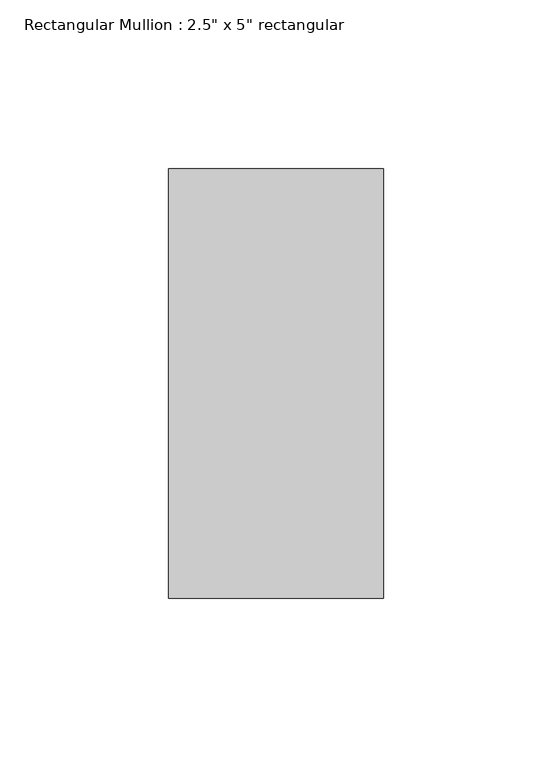
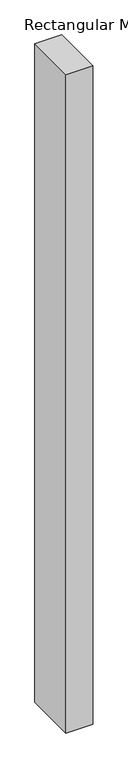
"""IFC4 building model written with IfcOpenShell, lengths in millimetres: member geometry."""

from ifc_helpers import new_model, si_unit, frame, origin, place, context, project, spatial, polyline, outline, extrude, source, transform, mapped, element, save


def member_61c652d3(model_context):
    return source(origin(), model_context, "Body", "SweptSolid", [
        extrude(outline(polyline([(0.0, 63.5), (0.0, -63.5), (-63.5, -63.5), (-63.5, 63.5), (0.0, 63.5)])), frame((0.0, 0.0, -1645.1858302), z_axis=(0.0, 0.0, 1.0), x_axis=(1.0, 0.0, 0.0)), (0.0, 0.0, 1.0), 1645.1858302),
    ])


if __name__ == "__main__":
    model = new_model("IFC4")
    model_context = context("Model", 3, world=origin())
    ifc_project = project(units=[si_unit("LENGTHUNIT", "METRE", prefix="MILLI")], contexts=[model_context])
    site = spatial("IfcSite", under=ifc_project)
    building = spatial("IfcBuilding", under=site)
    placement = place(None, origin())
    member_shape = member_61c652d3(model_context)
    element("IfcMember", 1, ObjectType="Rectangular Mullion : 2.5\" x 5\" rectangular", at=placement, inside=building, context=model_context, shape_type="MappedRepresentation", body=[
        mapped(member_shape, transform((0.0, 0.0, 0.0), x_axis=(1.0, 0.0, 0.0), y_axis=(0.0, 1.0, 0.0), z_axis=(0.0, 0.0, 1.0))),
    ])
    save(model, "model.ifc")

# Revit data of these elements
# Type "Rectangular Mullion : 2.5\" x 5\" rectangular"
#   built-in parameter 1007304 = 0.416667 (stored number, unit not read)
#   built-in parameter 1007301 = 0.104167 (stored number, unit not read)
#   built-in parameter 1007300 = 0.104167 (stored number, unit not read)
# Element 1 (IfcMember, "Rectangular Mullion : 2.5\" x 5\" rectangular")
#   Materials on its faces: "Aluminum"
# Materials
#   "Aluminum": class "Metal", colour RGB 247 247 247, transparency 0, Description = "Aluminum 6061", Cost = 0
